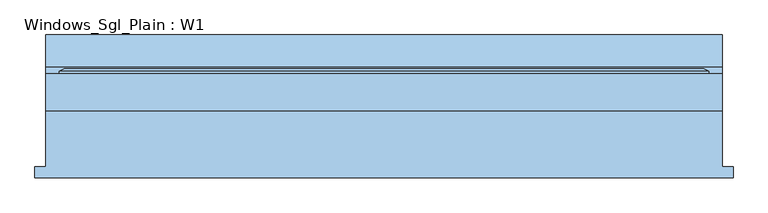
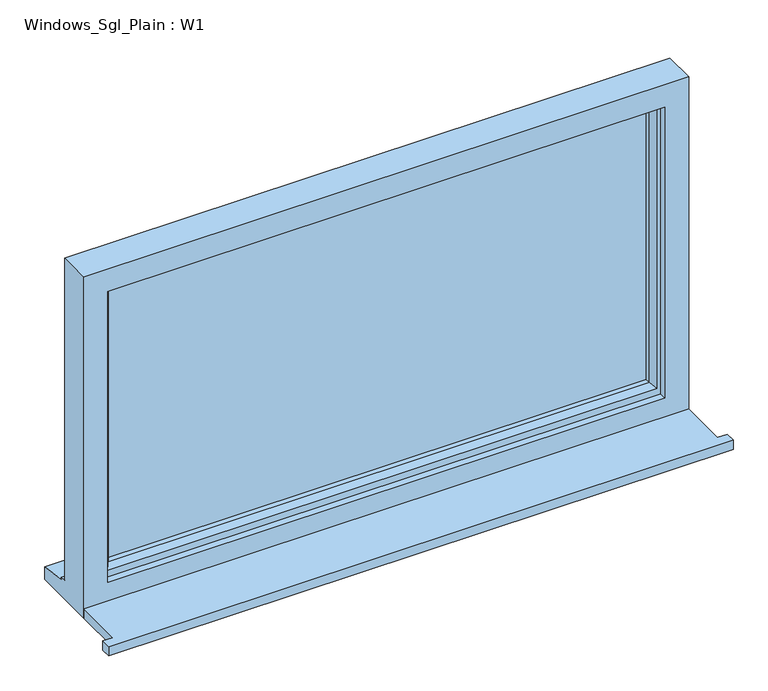
"""IFC4 building model written with IfcOpenShell, lengths in millimetres: window geometry, Windows_Sgl_Plain : W1."""

from ifc_helpers import new_model, si_unit, frame, origin, place, context, project, spatial, polyline, outline, extrude, faceted_brep, source, transform, mapped, element, save


def windows_sgl_plain_w1_a675e60d(model_context):
    return source(origin(), model_context, "Body", "SolidModel", [
        extrude(outline(polyline([(-787.0, -146.0834322), (-787.0, -121.0834322), (-762.0, -121.0834322), (-762.0, 4.9965678), (762.0, 4.9965678), (762.0, -121.0834322), (787.0, -121.0834322), (787.0, -146.0834322), (-787.0, -146.0834322)])), frame((0.0, 0.0, 1200.0), z_axis=(0.0, 0.0, 1.0), x_axis=(1.0, 0.0, 0.0)), (0.0, 0.0, 1.0), 25.0),
        faceted_brep([(-762.0, 4.9965678, 1200.0), (762.0, 4.9965678, 1200.0), (762.0, 4.9965678, 2110.0), (-762.0, 4.9965678, 2110.0), (-702.0, 4.9965678, 2050.0), (702.0, 4.9965678, 2050.0), (702.0, 4.9965678, 1275.0), (-702.0, 4.9965678, 1275.0), (-762.0, 87.9965678, 2110.0), (-762.0, 87.9965678, 1251.0), (-762.0, 102.9965678, 1249.68767), (-762.0, 102.9965678, 1244.7449676), (-762.0, 175.4965678, 1233.8088847), (-762.0, 175.4965678, 1200.0), (762.0, 87.9965678, 2110.0), (762.0, 87.9965678, 1251.0), (-722.0, 87.9965678, 2070.0), (-722.0, 87.9965678, 1263.0), (722.0, 87.9965678, 1263.0), (722.0, 87.9965678, 2070.0), (-722.0, 22.9965678, 2070.0), (-722.0, 22.9965678, 1263.0), (722.0, 22.9965678, 2070.0), (722.0, 22.9965678, 1263.0), (-702.0, 22.9965678, 2050.0), (-702.0, 22.9965678, 1275.0), (702.0, 22.9965678, 1275.0), (702.0, 22.9965678, 2050.0), (762.0, 175.4965678, 1200.0), (762.0, 175.4965678, 1233.8088847), (762.0, 102.9965678, 1244.7449676), (762.0, 102.9965678, 1249.68767)], [[[0, 1, 2, 3], [4, 5, 6, 7]], [[0, 3, 8, 9, 10, 11, 12, 13]], [[9, 8, 14, 15], [16, 17, 18, 19]], [[17, 16, 20, 21]], [[20, 22, 23, 21], [24, 25, 26, 27]], [[24, 4, 7, 25]], [[3, 2, 14, 8]], [[16, 19, 22, 20]], [[5, 4, 24, 27]], [[15, 14, 2, 1, 28, 29, 30, 31]], [[19, 18, 23, 22]], [[5, 27, 26, 6]], [[28, 1, 0, 13]], [[29, 28, 13, 12]], [[30, 29, 12, 11]], [[31, 30, 11, 10]], [[15, 31, 10, 9]], [[21, 23, 18, 17]], [[7, 6, 26, 25]]]),
        extrude(outline(polyline([(692.0, 51.9965678), (-692.0, 51.9965678), (-692.0, 75.9965678), (692.0, 75.9965678), (692.0, 51.9965678)])), frame((0.0, 0.0, 1293.0), z_axis=(0.0, 0.0, 1.0), x_axis=(1.0, 0.0, 0.0)), (0.0, 0.0, 1.0), 747.0),
        faceted_brep([(-732.0, 87.9965678, 2080.0), (-732.0, 93.7700705, 2080.0), (-732.0, 93.7700705, 1253.0), (-732.0, 87.9965678, 1253.0), (-722.0, 22.9965678, 2070.0), (-722.0, 87.9965678, 2070.0), (-722.0, 87.9965678, 1263.0), (-722.0, 22.9965678, 1263.0), (-682.0, 37.4894677, 2030.0), (-692.1480377, 22.9965678, 2040.1480377), (-692.1480377, 22.9965678, 1292.8519623), (-682.0, 37.4894677, 1303.0), (-682.0, 51.9965678, 2030.0), (-682.0, 51.9965678, 1303.0), (-692.0, 75.9965678, 2040.0), (-692.0, 51.9965678, 2040.0), (-692.0, 51.9965678, 1293.0), (-692.0, 75.9965678, 1293.0), (-682.0, 93.7700705, 2030.0), (-682.0, 75.9965678, 2030.0), (-682.0, 75.9965678, 1303.0), (-682.0, 93.7700705, 1303.0), (-699.4457548, 99.5435732, 2047.4457548), (-699.4457548, 99.5435732, 1285.5542452), (-721.2153903, 99.5435732, 2069.2153903), (-721.2153903, 99.5435732, 1263.7846097), (732.0, 93.7700705, 1253.0), (732.0, 87.9965678, 1253.0), (722.0, 87.9965678, 1263.0), (722.0, 22.9965678, 1263.0), (692.1480377, 22.9965678, 1292.8519623), (682.0, 37.4894677, 1303.0), (682.0, 51.9965678, 1303.0), (692.0, 51.9965678, 1293.0), (692.0, 75.9965678, 1293.0), (682.0, 75.9965678, 1303.0), (682.0, 93.7700705, 1303.0), (699.4457548, 99.5435732, 1285.5542452), (721.2153903, 99.5435732, 1263.7846097), (732.0, 93.7700705, 2080.0), (732.0, 87.9965678, 2080.0), (722.0, 87.9965678, 2070.0), (722.0, 22.9965678, 2070.0), (692.1480377, 22.9965678, 2040.1480377), (682.0, 37.4894677, 2030.0), (682.0, 51.9965678, 2030.0), (692.0, 51.9965678, 2040.0), (692.0, 75.9965678, 2040.0), (682.0, 75.9965678, 2030.0), (682.0, 93.7700705, 2030.0), (699.4457548, 99.5435732, 2047.4457548), (721.2153903, 99.5435732, 2069.2153903)], [[[0, 1, 2, 3]], [[4, 5, 6, 7]], [[8, 9, 10, 11]], [[12, 8, 11, 13]], [[14, 15, 16, 17]], [[18, 19, 20, 21]], [[22, 18, 21, 23]], [[1, 24, 25, 2]], [[3, 2, 26, 27]], [[7, 6, 28, 29]], [[11, 10, 30, 31]], [[13, 11, 31, 32]], [[17, 16, 33, 34]], [[21, 20, 35, 36]], [[23, 21, 36, 37]], [[2, 25, 38, 26]], [[27, 26, 39, 40]], [[29, 28, 41, 42]], [[31, 30, 43, 44]], [[32, 31, 44, 45]], [[34, 33, 46, 47]], [[36, 35, 48, 49]], [[37, 36, 49, 50]], [[26, 38, 51, 39]], [[40, 39, 1, 0]], [[3, 27, 40, 0], [5, 41, 28, 6]], [[42, 41, 5, 4]], [[7, 29, 42, 4], [9, 43, 30, 10]], [[44, 43, 9, 8]], [[45, 44, 8, 12]], [[15, 46, 33, 16], [13, 32, 45, 12]], [[47, 46, 15, 14]], [[17, 34, 47, 14], [19, 48, 35, 20]], [[49, 48, 19, 18]], [[50, 49, 18, 22]], [[24, 51, 38, 25], [23, 37, 50, 22]], [[39, 51, 24, 1]]]),
    ])


if __name__ == "__main__":
    model = new_model("IFC4")
    model_context = context("Model", 3, world=origin())
    ifc_project = project(units=[si_unit("LENGTHUNIT", "METRE", prefix="MILLI")], contexts=[model_context])
    site = spatial("IfcSite", under=ifc_project)
    building = spatial("IfcBuilding", under=site)
    placement = place(None, origin())
    windows_sgl_plain_w1_shape = windows_sgl_plain_w1_a675e60d(model_context)
    element("IfcWindow", 1, ObjectType="Windows_Sgl_Plain : W1", at=placement, inside=building, context=model_context, shape_type="MappedRepresentation", body=[
        mapped(windows_sgl_plain_w1_shape, transform((0.0, 0.0, 0.0), x_axis=(1.0, 0.0, 0.0), y_axis=(0.0, 1.0, 0.0), z_axis=(0.0, 0.0, 1.0))),
    ])
    save(model, "model.ifc")

# Revit data of these elements
# Type "Windows_Sgl_Plain : W1"
#   Type Mark = "60"
#   Operation = "SinglePanel"
#   Construction Type Id = "SGL"
#   Manufacturer = "Revit"
#   Keynote = "L10"
#   Analytic Construction = "Large single-glazed windows"
#   Wrap Layers (Ext) from Ext = 0.336286 ft
#   Wrap Layers (Int) from Ext = 0.582349 ft
#   Window Board Projection = 0.082021 ft
#   Window Board Extension = 0.082021 ft
#   Visual Light Transmittance = 0.9
#   Solar Heat Gain Coefficient = 0.86
#   Rough Width = 5.0 ft
#   Rough Height = 2.985564 ft
#   Height = 2.985564 ft
#   Width = 5.0 ft
#   Heat Transfer Coefficient (U) = 5.5617 W/(m²·K)
#   Glazing Thickness = 0.07874 ft
#   FrameOffset - External = 0.164042 ft
#   Frame Depth = 0.213255 ft
#   Default Head Height = 6.922572 ft
#   Cill Depth = 0.287073 ft
#   Cavity Closer Width = 0.164042 ft
#   Cavity Closer Offset from Ext = 0.336286 ft
#   Cavity Closer Depth = 0.278871 ft
#   Vis - Cavity Closers = yes
#   Define Thermal Properties by = 1
#   Material Trim = Window Frame
#   Material Glass = Glass
#   Material Frame = Window Frame
#   Wall Closure = (empty or 0)
# Element 1 (IfcWindow, "Windows_Sgl_Plain : W1")
#   Materials on its faces: "Window Frame", "Glass"
# Materials
#   "Window Frame": colour RGB 249 249 249, transparency 0, Keynote = "L10", Cost = 0
#   "Glass": class "Glass", colour RGB 0 128 192, transparency 0.9, Description = "Soda Lime Glass", Cost = 0
